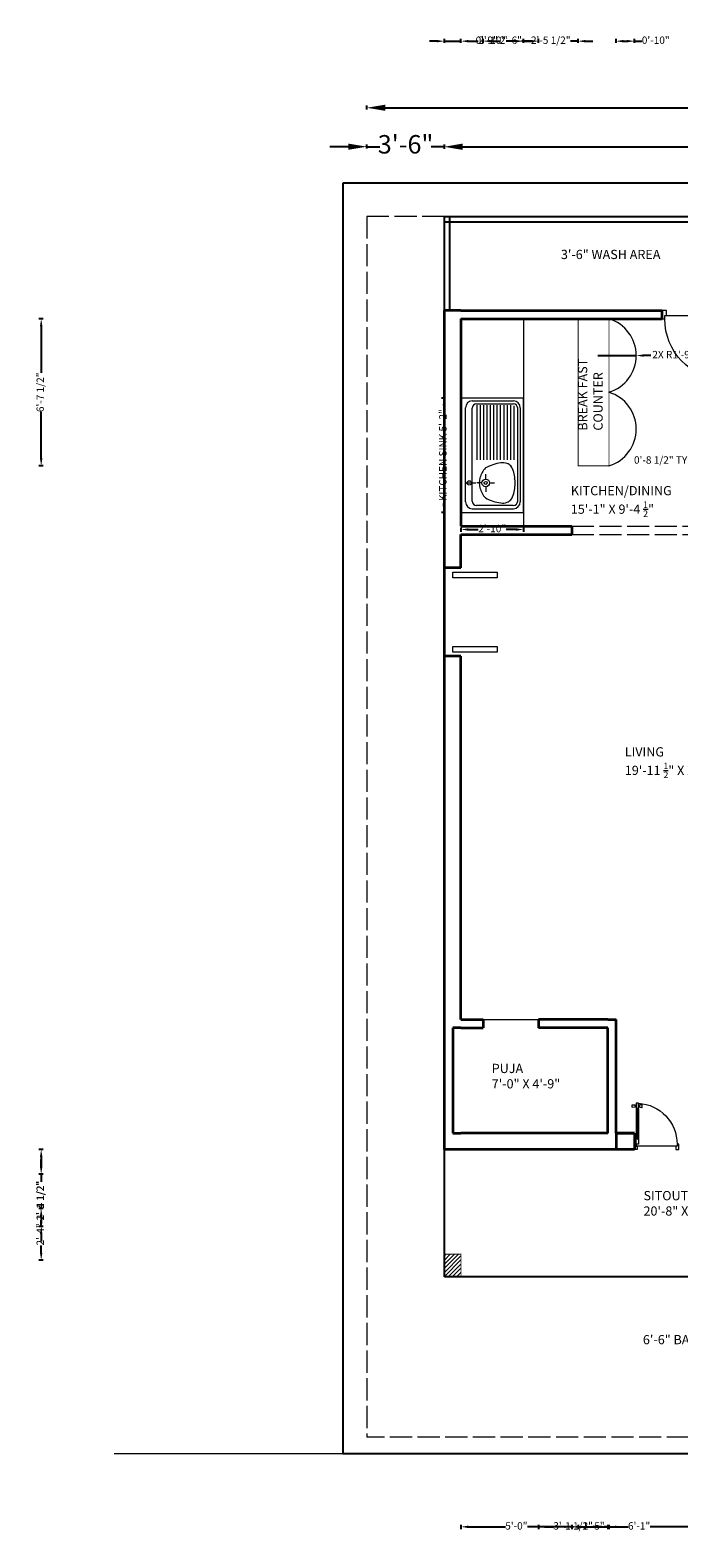
# Model space of a CAD drawing. Units: inches. Extents: x -638 to 186, y -762 to 59.
# Tile 1 of 31: x -638 to -287, y -759 to 59. Entities that reach past the tile are written whole.
import ezdxf

# ---------------------------------------------------------------- set-up
doc = ezdxf.new("R2010")
doc.units = ezdxf.units.IN
doc.linetypes.add('ACAD_ISO02W100', pattern=[15, 12, -3])
for name, color, linetype, lineweight in [('A-ANNO-DIMS', 2, 'Continuous', 18), ('A-AREA-IDEN', 1, 'Continuous', 18), ('A-COLS', 7, 'Continuous', 35), ('A-COLS-PATT', 1, 'Continuous', 13), ('A-DOOR', 3, 'Continuous', 18), ('A-FLOR-CASE', 1, 'Continuous', 18), ('A-FLOR-EDGE', 1, 'Continuous', 25), ('A-FLOR-FIXT', 9, 'Continuous', 18), ('A-FLOR-OVHD', 1, 'ACAD_ISO02W100', 18), ('A-WALL-OVHD', 1, 'ACAD_ISO02W100', 18), ('C-PROP', 7, 'Continuous', 25), ('C-ROAD', 7, 'Continuous', 18), ('txt', 7, 'Continuous', 18), ('wall', 7, 'Continuous', 35)]:
    doc.layers.add(name, color=color, linetype=linetype, lineweight=lineweight)
doc.styles.get("Standard").update_dxf_attribs({"font": 'arial.ttf'})
doc.dimstyles.new('ISO-25', dxfattribs={"dimtxt": 4, "dimasz": 4, "dimexe": 1.25, "dimexo": 0.625, "dimtad": 0, "dimlunit": 4, "dimtxsty": 'Standard', "dimcen": 2.5, "dimclrt": 256, "dimadec": 0, "dimazin": 0, "dimtfac": 1, "dimtmove": 0, "dimatfit": 3, "dimfxl": 1, "dimfxlon": 1, "dimarcsym": 0})

# ---------------------------------------------------------------- blocks, each defined once
blk = doc.blocks.new('19')
at = {"color": 0}
for p, q in [((4069.2, 13480.3), (4069.2, 13409.9)), ((4198.2, 13480.3), (4069.2, 13480.3)), ((4072.5, 13422.6), (4072.5, 13469.1)), ((4139, 13469.9), (4078.1, 13469.9)), ((4080.1, 13476.7), (4186.3, 13476.7)), ((4185.4, 13473.8), (4080.8, 13473.8)), ((4194, 13422.6), (4194, 13469.1)), ((4198.2, 13409.9), (4198.2, 13480.3)), ((4075.9, 13427.5), (4075.9, 13468.9)), ((4139, 13466), (4077.2, 13466)), ((4139, 13462.2), (4077.2, 13462.2)), ((4139, 13458.4), (4077.2, 13458.4)), ((4139, 13454.6), (4077.2, 13454.6)), ((4190.3, 13468.9), (4190.3, 13427.5)), ((4139, 13450.8), (4077.2, 13450.8)), ((4139, 13447), (4077.2, 13447)), ((4139, 13443.2), (4077.2, 13443.2)), ((4139, 13439.4), (4077.2, 13439.4)), ((4139, 13435.6), (4077.2, 13435.6)), ((4160.6, 13437.8), (4154.9, 13437.8)), ((4164.9, 13442.1), (4164.9, 13447.8)), ((4169.2, 13437.8), (4174.9, 13437.8)), ((4139, 13431.8), (4077.2, 13431.8)), ((4077.2, 13427.9), (4139, 13427.9)), ((4185.4, 13422.5), (4080.8, 13422.5)), ((4164.9, 13433.5), (4164.9, 13427.8)), ((4164.9, 13415.7), (4164.9, 13426.7)), ((4069.2, 13409.9), (4198.2, 13409.9)), ((4186.3, 13415), (4080.1, 13415))]:
    blk.add_line(p, q, dxfattribs=at)
for centre, radius in [((4164.9, 13437.8), 4.3), ((4164.9, 13437.8), 1.72), ((4164.9, 13419.2), 2.42)]:
    blk.add_circle(centre, radius, dxfattribs=at)
for points in [[(4080.1, 13476.7), (4075.9, 13476.7), (4072.5, 13473.3), (4072.5, 13469.1)], [(4080.8, 13473.8), (4078.1, 13473.8), (4075.9, 13471.6), (4075.9, 13468.9)], [(4160.4, 13470.6), (4155.2, 13470.4), (4150.2, 13468.9), (4145.7, 13466.1)], [(4162.1, 13470.8), (4161.6, 13470.7), (4161, 13470.6), (4160.5, 13470.4)], [(4169.4, 13470.6), (4167, 13471), (4164.6, 13471.1), (4162.1, 13470.8)], [(4184.1, 13466.1), (4179.7, 13468.9), (4174.6, 13470.4), (4169.4, 13470.6)], [(4190.3, 13468.9), (4190.3, 13471.6), (4188.1, 13473.8), (4185.4, 13473.8)], [(4194, 13469.1), (4194, 13473.3), (4190.5, 13476.7), (4186.3, 13476.7)], [(4143.1, 13461.8), (4142.2, 13459.6), (4141.9, 13457.2), (4142.4, 13454.9)], [(4142.4, 13454.9), (4143.2, 13448.8), (4145.1, 13442.9), (4148.1, 13437.5)], [(4145.7, 13466.1), (4144.5, 13464.9), (4143.6, 13463.4), (4143.1, 13461.8)], [(4181.8, 13437.5), (4184.8, 13442.9), (4186.7, 13448.8), (4187.5, 13454.9)], [(4186.7, 13461.8), (4186.2, 13463.4), (4185.3, 13464.9), (4184.1, 13466.1)], [(4187.5, 13454.9), (4187.9, 13457.2), (4187.7, 13459.6), (4186.7, 13461.8)], [(4148.1, 13437.5), (4151.2, 13434.5), (4155.1, 13432.4), (4159.3, 13431.3)], [(4170.6, 13431.3), (4174.8, 13432.4), (4178.7, 13434.5), (4181.8, 13437.5)], [(4072.5, 13422.6), (4072.5, 13418.4), (4075.9, 13415), (4080.1, 13415)], [(4075.9, 13427.5), (4075.9, 13424.7), (4078.1, 13422.5), (4080.8, 13422.5)], [(4159.3, 13431.3), (4163, 13430.2), (4166.9, 13430.2), (4170.6, 13431.3)], [(4185.4, 13422.5), (4188.1, 13422.5), (4190.3, 13424.7), (4190.3, 13427.5)], [(4186.3, 13415), (4190.5, 13415), (4194, 13418.4), (4194, 13422.6)]]:
    blk.add_open_spline(points, degree=3, dxfattribs=at)
blk = doc.blocks.new('*D8')
at = {"layer": 'A-ANNO-DIMS', "color": 0, "lineweight": -2, "transparency": 16777216}
for p, q in [((-465.53, -4.21), (-475.53, -4.21)), ((-455.53, -5.21), (-455.53, -2.96)), ((-455.53, -4.21), (-448.44, -4.21)), ((-413.53, -4.21), (-420.61, -4.21)), ((-413.53, -5.21), (-413.53, -2.96)), ((-403.53, -4.21), (-393.53, -4.21))]:
    blk.add_line(p, q, dxfattribs=at)
at = {"layer": 'A-ANNO-DIMS', "color": 0, "lineweight": 30, "transparency": 16777216}
for points in [[(-465.53, -2.54), (-465.53, -5.87), (-455.53, -4.21)], [(-403.53, -2.54), (-403.53, -5.87), (-413.53, -4.21)]]:
    blk.add_solid(points, dxfattribs=at)
at = {"layer": 'Defpoints', "color": 0, "lineweight": 30, "transparency": 16777216}
for p in [(-413.53, -4.21), (-455.53, -42.03), (-413.53, -42.03)]:
    blk.add_point(p, dxfattribs=at)
at = {"layer": 'A-ANNO-DIMS', "color": 0, "transparency": 16777216, "insert": (-434.53, -4.21), "char_height": 10, "attachment_point": 5}
blk.add_mtext('3\'-6"', dxfattribs=at)
blk = doc.blocks.new('*D9')
at = {"layer": 'A-ANNO-DIMS', "color": 0, "lineweight": -2, "transparency": 16777216}
for p, q in [((-413.53, -5.3), (-413.53, -3.05)), ((-403.53, -4.3), (-219.32, -4.3)), ((0.47, -4.3), (-183.73, -4.3)), ((10.47, -5.3), (10.47, -3.05))]:
    blk.add_line(p, q, dxfattribs=at)
at = {"layer": 'A-ANNO-DIMS', "color": 0, "lineweight": 30, "transparency": 16777216}
for points in [[(-403.53, -2.64), (-403.53, -5.97), (-413.53, -4.3)], [(0.47, -2.64), (0.47, -5.97), (10.47, -4.3)]]:
    blk.add_solid(points, dxfattribs=at)
at = {"layer": 'Defpoints', "color": 0, "lineweight": 30, "transparency": 16777216}
for p in [(10.47, -4.3), (-413.53, -42.03), (10.47, -42.03)]:
    blk.add_point(p, dxfattribs=at)
at = {"layer": 'A-ANNO-DIMS', "color": 0, "transparency": 16777216, "insert": (-201.53, -4.3), "char_height": 10, "attachment_point": 5}
blk.add_mtext('35\'-4"', dxfattribs=at)
blk = doc.blocks.new('*D11')
at = {"layer": 'A-ANNO-DIMS', "color": 0, "lineweight": -2, "transparency": 16777216}
for p, q in [((-455.53, 15.89), (-455.53, 18.14)), ((-445.53, 16.89), (-231.53, 16.89)), ((18.47, 16.89), (-195.52, 16.89)), ((28.47, 15.89), (28.47, 18.14))]:
    blk.add_line(p, q, dxfattribs=at)
at = {"layer": 'A-ANNO-DIMS', "color": 0, "lineweight": 30, "transparency": 16777216}
for points in [[(-445.53, 18.56), (-445.53, 15.23), (-455.53, 16.89)], [(18.47, 18.56), (18.47, 15.23), (28.47, 16.89)]]:
    blk.add_solid(points, dxfattribs=at)
at = {"layer": 'Defpoints', "color": 0, "lineweight": 30, "transparency": 16777216}
for p in [(28.47, 16.89), (-455.53, -42.03), (28.47, -42.03)]:
    blk.add_point(p, dxfattribs=at)
at = {"layer": 'A-ANNO-DIMS', "color": 0, "transparency": 16777216, "insert": (-213.53, 16.89), "char_height": 10, "attachment_point": 5}
blk.add_mtext('40\'-4"', dxfattribs=at)
blk = doc.blocks.new('DOOR-SWING-36IN')
for p, q in [((35.54, 35.1), (4.05, 35.09)), ((3.16, 4.5), (3.16, 28.79)), ((3.95, 4.05), (3.94, 29.24)), ((4.06, 4.05), (4.06, 29.24)), ((4.18, 4.05), (4.17, 29.24)), ((4.96, 4.5), (4.96, 28.79))]:
    blk.add_line(p, q)
for points in [[(3.16, 33.29), (3.15, 35.09), (4.05, 35.09), (4.05, 37.78), (1.8, 37.78), (1.81, 33.29), (3.16, 33.29)], [(4.28, 28.79), (4.96, 28.79), (4.95, 33.29), (3.16, 33.29), (3.16, 28.79), (3.83, 28.79), (3.83, 29.24), (4.28, 29.24), (4.28, 28.79)], [(36.44, 33.3), (36.44, 35.1), (35.54, 35.1), (35.54, 37.79), (37.79, 37.8), (37.79, 33.3), (36.44, 33.3)], [(4.29, 4.5), (4.96, 4.5), (4.96, 0), (3.17, 0), (3.16, 4.5), (3.84, 4.5), (3.84, 4.05), (4.29, 4.05), (4.29, 4.5)]]:
    blk.add_lwpolyline(points)
for points in [[(2.05, 3.17), (0.25, 3.35, 0.443716), (0, 3.12), (0, 1.37, 0.443716), (0.25, 1.15), (2.05, 1.33, 0.385314), (2.25, 1.55), (2.25, 2.94, 0.385314)], [(6.08, 3.17), (7.88, 3.35, -0.443716), (8.13, 3.13), (8.13, 1.37, -0.443716), (7.88, 1.15), (6.08, 1.33, -0.385314), (5.88, 1.55), (5.88, 2.95, -0.385314)]]:
    blk.add_lwpolyline(points, format="xyb", close=True)
for points in [[(3.16, 2.47), (2.25, 2.47), (2.25, 2.02), (3.17, 2.02)], [(4.96, 2.47), (5.88, 2.47), (5.88, 2.03), (4.96, 2.02)]]:
    blk.add_lwpolyline(points, close=True)
for centre, radius, start, end in [((3.06, 33.32), 33.38, 273.26531, 359.95298), ((3.92, 28.83), 0.371, 186.45223, 273.3078), ((4.19, 28.83), 0.371, 266.72821, 353.58377), ((3.93, 4.46), 0.371, 86.72821, 173.58377), ((4.2, 4.46), 0.371, 6.45223, 93.3078)]:
    blk.add_arc(centre, radius, start, end)
blk = doc.blocks.new('DOOR-ENTRY-24IN-LEAF')
for p, q in [((21.85, 22.14), (21.85, 5.99)), ((22.38, 22.44), (22.37, 5.69)), ((22.45, 22.44), (22.45, 5.69)), ((22.53, 22.44), (22.52, 5.69)), ((23.05, 22.14), (23.04, 5.99)), ((1.5, 1.8), (22.44, 1.8))]:
    blk.add_line(p, q)
for points in [[(22.3, 22.14), (21.85, 22.14), (21.85, 25.14), (23.05, 25.14), (23.05, 22.14), (22.6, 22.14), (22.6, 22.44), (22.3, 22.44), (22.3, 22.14)], [(0.9, 3), (0.9, 1.8), (1.5, 1.8), (1.5, 0.01), (0, 0.01), (0, 3), (0.9, 3)], [(22.3, 5.99), (21.85, 5.99), (21.85, 2.99), (23.04, 2.99), (23.04, 5.99), (22.59, 5.99), (22.59, 5.69), (22.3, 5.69), (22.3, 5.99)], [(23.04, 2.99), (23.04, 1.8), (22.44, 1.8), (22.44, 0), (23.94, 0), (23.94, 2.99), (23.04, 2.99)]]:
    blk.add_lwpolyline(points)
for points in [[(21.11, 23.03), (19.91, 22.91, -0.443716), (19.75, 23.06), (19.75, 24.22, -0.443716), (19.91, 24.37), (21.11, 24.25, -0.385314), (21.24, 24.1), (21.24, 23.18, -0.385314)], [(23.79, 23.03), (24.99, 22.91, 0.443716), (25.15, 23.06), (25.16, 24.22, 0.443716), (24.99, 24.37), (23.79, 24.25, 0.385314), (23.66, 24.1), (23.66, 23.18, 0.385314)]]:
    blk.add_lwpolyline(points, format="xyb", close=True)
for points in [[(21.85, 23.49), (21.24, 23.49), (21.24, 23.79), (21.85, 23.79)], [(23.05, 23.49), (23.66, 23.49), (23.66, 23.79), (23.05, 23.79)]]:
    blk.add_lwpolyline(points, close=True)
for centre, radius, start, end in [((23.1, 2.97), 22.21, 93.2293, 179.91697), ((22.36, 22.17), 0.247, 186.41623, 273.27179), ((22.54, 22.17), 0.247, 266.6922, 353.54777), ((22.36, 5.96), 0.247, 86.6922, 173.54777), ((22.53, 5.96), 0.247, 6.41623, 93.27179)]:
    blk.add_arc(centre, radius, start, end)
blk = doc.blocks.new('*D22')
at = {"layer": 'A-ANNO-DIMS', "color": 0, "lineweight": -2, "transparency": 16777216}
for p, q in [((-272.41, -174.6), (-276.41, -174.6)), ((-268.41, -173.71), (-268.41, -175.85)), ((-260.07, -174.6), (-268.41, -174.6)), ((-260.07, -173.71), (-260.07, -175.85)), ((-256.07, -174.6), (-252.07, -174.6))]:
    blk.add_line(p, q, dxfattribs=at)
at = {"layer": 'A-ANNO-DIMS', "color": 0, "lineweight": 30, "transparency": 16777216}
for points in [[(-272.41, -173.93), (-272.41, -175.26), (-268.41, -174.6)], [(-256.07, -173.93), (-256.07, -175.26), (-260.07, -174.6)]]:
    blk.add_solid(points, dxfattribs=at)
at = {"layer": 'Defpoints', "color": 0, "lineweight": 30, "transparency": 16777216}
for p in [(-268.41, -173.09), (-268.41, -174.6), (-260.07, -173.09)]:
    blk.add_point(p, dxfattribs=at)
at = {"layer": 'A-ANNO-DIMS', "transparency": 16777216, "insert": (-293.89, -174.6), "char_height": 4, "attachment_point": 5, "rotation": 360}
blk.add_mtext('0\'-8 1/2" TYP.', dxfattribs=at)
blk = doc.blocks.new('*D33')
at = {"layer": 'A-ANNO-DIMS', "color": 0, "lineweight": -2, "transparency": 16777216}
for p, q in [((-412.83, -140.48), (-415.08, -140.48)), ((-413.83, -144.48), (-413.83, -145.3)), ((-412.83, -202.49), (-415.08, -202.49)), ((-413.83, -198.49), (-413.83, -197.68))]:
    blk.add_line(p, q, dxfattribs=at)
at = {"layer": 'A-ANNO-DIMS', "color": 0, "lineweight": 30, "transparency": 16777216}
for points in [[(-414.49, -144.48), (-413.16, -144.48), (-413.83, -140.48)], [(-414.49, -198.49), (-413.16, -198.49), (-413.83, -202.49)]]:
    blk.add_solid(points, dxfattribs=at)
at = {"layer": 'Defpoints', "color": 0, "lineweight": 30, "transparency": 16777216}
for p in [(-404.53, -140.48), (-413.83, -202.49), (-404.53, -202.49)]:
    blk.add_point(p, dxfattribs=at)
at = {"layer": 'A-ANNO-DIMS', "transparency": 16777216, "insert": (-413.83, -171.49), "char_height": 4, "attachment_point": 5, "rotation": 90}
blk.add_mtext('KITCHEN SINK 5\'-2"', dxfattribs=at)
blk = doc.blocks.new('*D34')
at = {"layer": 'A-ANNO-DIMS', "color": 0, "lineweight": -2, "transparency": 16777216}
for p, q in [((-404.53, -210.79), (-404.53, -213.04)), ((-400.53, -211.79), (-395.15, -211.79)), ((-374.71, -211.79), (-380.09, -211.79)), ((-370.71, -210.79), (-370.71, -213.04))]:
    blk.add_line(p, q, dxfattribs=at)
at = {"layer": 'A-ANNO-DIMS', "color": 0, "lineweight": 30, "transparency": 16777216}
for points in [[(-400.53, -211.12), (-400.53, -212.46), (-404.53, -211.79)], [(-374.71, -211.12), (-374.71, -212.46), (-370.71, -211.79)]]:
    blk.add_solid(points, dxfattribs=at)
at = {"layer": 'Defpoints', "color": 0, "lineweight": 30, "transparency": 16777216}
for p in [(-404.53, -202.49), (-370.71, -202.49), (-370.71, -211.79)]:
    blk.add_point(p, dxfattribs=at)
at = {"layer": 'A-ANNO-DIMS', "transparency": 16777216, "insert": (-387.62, -211.79), "char_height": 4, "attachment_point": 5}
blk.add_mtext('2\'-10"', dxfattribs=at)
blk = doc.blocks.new('*D37')
at = {"layer": 'A-ANNO-DIMS', "color": 0, "lineweight": -2, "transparency": 16777216}
for p, q in [((182.66, -232.53), (184.91, -232.53)), ((183.66, -236.53), (183.66, -250.51)), ((183.66, -276.53), (183.66, -262.56)), ((182.66, -280.53), (184.91, -280.53))]:
    blk.add_line(p, q, dxfattribs=at)
at = {"layer": 'A-ANNO-DIMS', "color": 0, "lineweight": 30, "transparency": 16777216}
for points in [[(183, -236.53), (184.33, -236.53), (183.66, -232.53)], [(183, -276.53), (184.33, -276.53), (183.66, -280.53)]]:
    blk.add_solid(points, dxfattribs=at)
at = {"layer": 'Defpoints', "color": 0, "lineweight": 30, "transparency": 16777216}
for p in [(-404.53, -232.53), (-404.53, -280.53), (183.66, -280.53)]:
    blk.add_point(p, dxfattribs=at)
at = {"layer": 'A-ANNO-DIMS', "transparency": 16777216, "insert": (183.66, -256.53), "char_height": 4, "attachment_point": 5, "rotation": 90}
blk.add_mtext('4\'-0"', dxfattribs=at)
blk = doc.blocks.new('*D38')
at = {"layer": 'A-ANNO-DIMS', "color": 0, "lineweight": -2, "transparency": 16777216}
for p, q in [((182.66, -280.53), (184.91, -280.53)), ((183.66, -284.53), (183.66, -371.73)), ((183.66, -473.53), (183.66, -386.34)), ((182.66, -477.53), (184.91, -477.53))]:
    blk.add_line(p, q, dxfattribs=at)
at = {"layer": 'A-ANNO-DIMS', "color": 0, "lineweight": 30, "transparency": 16777216}
for points in [[(183, -284.53), (184.33, -284.53), (183.66, -280.53)], [(183, -473.53), (184.33, -473.53), (183.66, -477.53)]]:
    blk.add_solid(points, dxfattribs=at)
at = {"layer": 'Defpoints', "color": 0, "lineweight": 30, "transparency": 16777216}
for p in [(-404.53, -280.53), (-404.53, -477.53), (183.66, -477.53)]:
    blk.add_point(p, dxfattribs=at)
at = {"layer": 'A-ANNO-DIMS', "transparency": 16777216, "insert": (183.66, -379.03), "char_height": 4, "attachment_point": 5, "rotation": 90}
blk.add_mtext('16\'-5"', dxfattribs=at)
blk = doc.blocks.new('*D39')
at = {"layer": 'A-ANNO-DIMS', "color": 0, "lineweight": -2, "transparency": 16777216}
for p, q in [((-344.53, -751.58), (-344.53, -753.83)), ((-271.53, -751.58), (-271.53, -753.83)), ((-340.53, -752.58), (-313.98, -752.58)), ((-275.53, -752.58), (-302.07, -752.58))]:
    blk.add_line(p, q, dxfattribs=at)
at = {"layer": 'A-ANNO-DIMS', "color": 0, "lineweight": 30, "transparency": 16777216}
for points in [[(-340.53, -751.92), (-340.53, -753.25), (-344.53, -752.58)], [(-275.53, -751.92), (-275.53, -753.25), (-271.53, -752.58)]]:
    blk.add_solid(points, dxfattribs=at)
at = {"layer": 'Defpoints', "color": 0, "lineweight": 30, "transparency": 16777216}
for p in [(-344.53, -214.53), (-271.53, -214.53), (-271.53, -752.58)]:
    blk.add_point(p, dxfattribs=at)
at = {"layer": 'A-ANNO-DIMS', "transparency": 16777216, "insert": (-308.03, -752.58), "char_height": 4, "attachment_point": 5}
blk.add_mtext('6\'-1"', dxfattribs=at)
blk = doc.blocks.new('*D40')
at = {"layer": 'A-ANNO-DIMS', "color": 0, "lineweight": -2, "transparency": 16777216}
for p, q in [((-404.53, -751.58), (-404.53, -753.83)), ((-344.53, -751.58), (-344.53, -753.83)), ((-400.53, -752.58), (-380.47, -752.58)), ((-348.53, -752.58), (-368.58, -752.58))]:
    blk.add_line(p, q, dxfattribs=at)
at = {"layer": 'A-ANNO-DIMS', "color": 0, "lineweight": 30, "transparency": 16777216}
for points in [[(-400.53, -751.92), (-400.53, -753.25), (-404.53, -752.58)], [(-348.53, -751.92), (-348.53, -753.25), (-344.53, -752.58)]]:
    blk.add_solid(points, dxfattribs=at)
at = {"layer": 'Defpoints', "color": 0, "lineweight": 30, "transparency": 16777216}
for p in [(-404.53, -214.53), (-344.53, -214.53), (-344.53, -752.58)]:
    blk.add_point(p, dxfattribs=at)
at = {"layer": 'A-ANNO-DIMS', "transparency": 16777216, "insert": (-374.53, -752.58), "char_height": 4, "attachment_point": 5}
blk.add_mtext('5\'-0"', dxfattribs=at)
blk = doc.blocks.new('*D41')
at = {"layer": 'A-ANNO-DIMS', "color": 0, "lineweight": -2, "transparency": 16777216}
for p, q in [((-392.53, 52.02), (-392.53, 54.27)), ((-388.53, 53.02), (-383.5, 53.02)), ((-366.53, 53.02), (-371.55, 53.02)), ((-362.53, 52.02), (-362.53, 54.27))]:
    blk.add_line(p, q, dxfattribs=at)
at = {"layer": 'A-ANNO-DIMS', "color": 0, "lineweight": 30, "transparency": 16777216}
for points in [[(-388.53, 53.68), (-388.53, 52.35), (-392.53, 53.02)], [(-366.53, 53.68), (-366.53, 52.35), (-362.53, 53.02)]]:
    blk.add_solid(points, dxfattribs=at)
at = {"layer": 'Defpoints', "color": 0, "lineweight": 30, "transparency": 16777216}
for p in [(-362.53, 53.02), (-392.53, -477.53), (-362.53, -477.53)]:
    blk.add_point(p, dxfattribs=at)
at = {"layer": 'A-ANNO-DIMS', "transparency": 16777216, "insert": (-377.53, 53.02), "char_height": 4, "attachment_point": 5}
blk.add_mtext('2\'-6"', dxfattribs=at)
blk = doc.blocks.new('*D42')
at = {"layer": 'A-ANNO-DIMS', "color": 0, "lineweight": -2, "transparency": 16777216}
for p, q in [((-362.53, -751.58), (-362.53, -753.83)), ((-325.03, -751.58), (-325.03, -753.83)), ((-358.53, -752.58), (-354.38, -752.58)), ((-329.03, -752.58), (-333.18, -752.58))]:
    blk.add_line(p, q, dxfattribs=at)
at = {"layer": 'A-ANNO-DIMS', "color": 0, "lineweight": 30, "transparency": 16777216}
for points in [[(-358.53, -751.92), (-358.53, -753.25), (-362.53, -752.58)], [(-329.03, -751.92), (-329.03, -753.25), (-325.03, -752.58)]]:
    blk.add_solid(points, dxfattribs=at)
at = {"layer": 'Defpoints', "color": 0, "lineweight": 30, "transparency": 16777216}
for p in [(-362.53, -482.03), (-325.03, -482.03), (-325.03, -752.58)]:
    blk.add_point(p, dxfattribs=at)
at = {"layer": 'A-ANNO-DIMS', "transparency": 16777216, "insert": (-343.78, -752.58), "char_height": 4, "attachment_point": 5}
blk.add_mtext('3\'-1 1/2"', dxfattribs=at)
blk = doc.blocks.new('*D43')
at = {"layer": 'A-ANNO-DIMS', "color": 0, "lineweight": -2, "transparency": 16777216}
for p, q in [((-320.53, 52.02), (-320.53, 54.27)), ((-316.53, 53.02), (-314.53, 53.02)), ((-310.53, 52.02), (-310.53, 54.27)), ((-310.53, 53.02), (-306.53, 53.02))]:
    blk.add_line(p, q, dxfattribs=at)
at = {"layer": 'A-ANNO-DIMS', "color": 0, "lineweight": 30, "transparency": 16777216}
for points in [[(-316.53, 53.68), (-316.53, 52.35), (-320.53, 53.02)], [(-314.53, 53.68), (-314.53, 52.35), (-310.53, 53.02)]]:
    blk.add_solid(points, dxfattribs=at)
at = {"layer": 'Defpoints', "color": 0, "lineweight": 30, "transparency": 16777216}
for p in [(-310.53, 53.02), (-320.53, -539.03), (-310.53, -539.03)]:
    blk.add_point(p, dxfattribs=at)
at = {"layer": 'A-ANNO-DIMS', "transparency": 16777216, "insert": (-299.03, 53.02), "char_height": 4, "attachment_point": 5}
blk.add_mtext('0\'-10"', dxfattribs=at)
blk = doc.blocks.new('*D44')
at = {"layer": 'A-ANNO-DIMS', "color": 0, "lineweight": -2, "transparency": 16777216}
for p, q in [((-417.53, 53.02), (-421.53, 53.02)), ((-413.53, 52.02), (-413.53, 54.27)), ((-413.53, 53.02), (-404.53, 53.02)), ((-404.53, 52.02), (-404.53, 54.27)), ((-400.53, 53.02), (-396.53, 53.02))]:
    blk.add_line(p, q, dxfattribs=at)
at = {"layer": 'A-ANNO-DIMS', "color": 0, "lineweight": 30, "transparency": 16777216}
for points in [[(-417.53, 53.68), (-417.53, 52.35), (-413.53, 53.02)], [(-400.53, 53.68), (-400.53, 52.35), (-404.53, 53.02)]]:
    blk.add_solid(points, dxfattribs=at)
at = {"layer": 'Defpoints', "color": 0, "lineweight": 30, "transparency": 16777216}
for p in [(-404.53, 53.02), (-413.53, -93.03), (-404.53, -97.53)]:
    blk.add_point(p, dxfattribs=at)
at = {"layer": 'A-ANNO-DIMS', "transparency": 16777216, "insert": (-390.58, 53.02), "char_height": 4, "attachment_point": 5}
blk.add_mtext('0\'-9"', dxfattribs=at)
blk = doc.blocks.new('*D45')
at = {"layer": 'A-ANNO-DIMS', "color": 0, "lineweight": -2, "transparency": 16777216}
for p, q in [((-374.7, 53.02), (-378.7, 53.02)), ((-370.7, 52.02), (-370.7, 54.27)), ((-370.7, 53.02), (-366.54, 53.02)), ((-341.11, 53.02), (-345.27, 53.02)), ((-341.11, 52.02), (-341.11, 54.27)), ((-337.11, 53.02), (-333.11, 53.02))]:
    blk.add_line(p, q, dxfattribs=at)
at = {"layer": 'A-ANNO-DIMS', "color": 0, "lineweight": 30, "transparency": 16777216}
for points in [[(-374.7, 53.68), (-374.7, 52.35), (-370.7, 53.02)], [(-337.11, 53.68), (-337.11, 52.35), (-341.11, 53.02)]]:
    blk.add_solid(points, dxfattribs=at)
at = {"layer": 'Defpoints', "color": 0, "lineweight": 30, "transparency": 16777216}
for p in [(-341.11, 53.02), (-370.7, -97.53), (-341.11, -97.53)]:
    blk.add_point(p, dxfattribs=at)
at = {"layer": 'A-ANNO-DIMS', "transparency": 16777216, "insert": (-355.9, 53.02), "char_height": 4, "attachment_point": 5}
blk.add_mtext('2\'-5 1/2"', dxfattribs=at)
blk = doc.blocks.new('*D46')
at = {"layer": 'A-ANNO-DIMS', "color": 0, "lineweight": -2, "transparency": 16777216}
for p, q in [((-630.93, -97.53), (-633.18, -97.53)), ((-631.93, -101.53), (-631.93, -126.78)), ((-631.93, -173.25), (-631.93, -148)), ((-630.93, -177.25), (-633.18, -177.25))]:
    blk.add_line(p, q, dxfattribs=at)
at = {"layer": 'A-ANNO-DIMS', "color": 0, "lineweight": 30, "transparency": 16777216}
for points in [[(-632.59, -101.53), (-631.26, -101.53), (-631.93, -97.53)], [(-632.59, -173.25), (-631.26, -173.25), (-631.93, -177.25)]]:
    blk.add_solid(points, dxfattribs=at)
at = {"layer": 'Defpoints', "color": 0, "lineweight": 30, "transparency": 16777216}
for p in [(-341.11, -97.53), (-631.93, -177.25), (-341.11, -177.25)]:
    blk.add_point(p, dxfattribs=at)
at = {"layer": 'A-ANNO-DIMS', "transparency": 16777216, "insert": (-631.93, -137.39), "char_height": 4, "attachment_point": 5, "rotation": 90}
blk.add_mtext('6\'-7 1/2"', dxfattribs=at)
blk = doc.blocks.new('*D47')
at = {"layer": 'A-ANNO-DIMS', "color": 0, "lineweight": -2, "transparency": 16777216}
for p, q in [((-341.11, -751.58), (-341.11, -753.83)), ((-324.35, -751.58), (-324.35, -753.83)), ((-345.11, -752.58), (-349.11, -752.58)), ((-341.11, -752.58), (-338.48, -752.58)), ((-324.35, -752.58), (-326.97, -752.58)), ((-320.35, -752.58), (-316.35, -752.58))]:
    blk.add_line(p, q, dxfattribs=at)
at = {"layer": 'A-ANNO-DIMS', "color": 0, "lineweight": 30, "transparency": 16777216}
for points in [[(-345.11, -751.92), (-345.11, -753.25), (-341.11, -752.58)], [(-320.35, -751.92), (-320.35, -753.25), (-324.35, -752.58)]]:
    blk.add_solid(points, dxfattribs=at)
at = {"layer": 'Defpoints', "color": 0, "lineweight": 30, "transparency": 16777216}
for p in [(-341.11, -177.25), (-324.35, -177.25), (-324.35, -752.58)]:
    blk.add_point(p, dxfattribs=at)
at = {"layer": 'A-ANNO-DIMS', "transparency": 16777216, "insert": (-332.73, -752.58), "char_height": 4, "attachment_point": 5}
blk.add_mtext('1\'-5"', dxfattribs=at)
blk = doc.blocks.new('*D50')
at = {"layer": 'A-ANNO-DIMS', "color": 0, "lineweight": -2, "transparency": 16777216}
for p, q in [((-631.93, -557.43), (-631.93, -553.43)), ((-630.93, -561.43), (-633.18, -561.43)), ((-631.93, -561.43), (-631.93, -564.98)), ((-631.93, -589.8), (-631.93, -586.25)), ((-630.93, -589.8), (-633.18, -589.8)), ((-631.93, -593.8), (-631.93, -597.8))]:
    blk.add_line(p, q, dxfattribs=at)
at = {"layer": 'A-ANNO-DIMS', "color": 0, "lineweight": 30, "transparency": 16777216}
for points in [[(-632.59, -557.43), (-631.26, -557.43), (-631.93, -561.43)], [(-632.59, -593.8), (-631.26, -593.8), (-631.93, -589.8)]]:
    blk.add_solid(points, dxfattribs=at)
at = {"layer": 'Defpoints', "color": 0, "lineweight": 30, "transparency": 16777216}
for p in [(-156.03, -561.43), (-631.93, -589.8), (-156.03, -589.8)]:
    blk.add_point(p, dxfattribs=at)
at = {"layer": 'A-ANNO-DIMS', "transparency": 16777216, "insert": (-631.93, -575.62), "char_height": 4, "attachment_point": 5, "rotation": 90}
blk.add_mtext('2\'-4 1/2"', dxfattribs=at)
blk = doc.blocks.new('*D52')
at = {"layer": 'A-ANNO-DIMS', "color": 0, "lineweight": -2, "transparency": 16777216}
for p, q in [((-630.93, -580.03), (-633.18, -580.03)), ((-631.93, -584.03), (-631.93, -588.06)), ((-631.93, -604.03), (-631.93, -600.01)), ((-630.93, -608.03), (-633.18, -608.03))]:
    blk.add_line(p, q, dxfattribs=at)
at = {"layer": 'A-ANNO-DIMS', "color": 0, "lineweight": 30, "transparency": 16777216}
for points in [[(-632.59, -584.03), (-631.26, -584.03), (-631.93, -580.03)], [(-632.59, -604.03), (-631.26, -604.03), (-631.93, -608.03)]]:
    blk.add_solid(points, dxfattribs=at)
at = {"layer": 'Defpoints', "color": 0, "lineweight": 30, "transparency": 16777216}
for p in [(-29.91, -580.03), (-631.93, -608.03), (-40.41, -608.03)]:
    blk.add_point(p, dxfattribs=at)
at = {"layer": 'A-ANNO-DIMS', "transparency": 16777216, "insert": (-631.93, -594.03), "char_height": 4, "attachment_point": 5, "rotation": 90}
blk.add_mtext('2\'-4"', dxfattribs=at)
blk = doc.blocks.new('*D54')
at = {"layer": 'A-ANNO-DIMS', "color": 0, "lineweight": -2, "transparency": 16777216}
for p, q in [((-404.53, 52.02), (-404.53, 54.27)), ((-400.53, 53.02), (-395.14, 53.02)), ((-374.7, 53.02), (-380.08, 53.02)), ((-370.7, 52.02), (-370.7, 54.27))]:
    blk.add_line(p, q, dxfattribs=at)
at = {"layer": 'A-ANNO-DIMS', "color": 0, "lineweight": 30, "transparency": 16777216}
for points in [[(-400.53, 53.68), (-400.53, 52.35), (-404.53, 53.02)], [(-374.7, 53.68), (-374.7, 52.35), (-370.7, 53.02)]]:
    blk.add_solid(points, dxfattribs=at)
at = {"layer": 'Defpoints', "color": 0, "lineweight": 30, "transparency": 16777216}
for p in [(-370.7, 53.02), (-404.53, -97.53), (-370.7, -97.53)]:
    blk.add_point(p, dxfattribs=at)
at = {"layer": 'A-ANNO-DIMS', "transparency": 16777216, "insert": (-387.61, 53.02), "char_height": 4, "attachment_point": 5}
blk.add_mtext('2\'-10"', dxfattribs=at)
blk = doc.blocks.new('*D57')
at = {"layer": 'A-ANNO-DIMS', "color": 0, "lineweight": -2, "transparency": 16777216}
for p, q in [((-630.93, -548.03), (-633.18, -548.03)), ((-631.93, -552.03), (-631.93, -557.43)), ((-630.93, -561.43), (-633.18, -561.43)), ((-631.93, -561.43), (-631.93, -565.43))]:
    blk.add_line(p, q, dxfattribs=at)
at = {"layer": 'A-ANNO-DIMS', "color": 0, "lineweight": 30, "transparency": 16777216}
for points in [[(-632.59, -552.03), (-631.26, -552.03), (-631.93, -548.03)], [(-632.59, -557.43), (-631.26, -557.43), (-631.93, -561.43)]]:
    blk.add_solid(points, dxfattribs=at)
at = {"layer": 'Defpoints', "color": 0, "lineweight": 30, "transparency": 16777216}
for p in [(-156.03, -548.03), (-631.93, -561.43), (-156.03, -561.43)]:
    blk.add_point(p, dxfattribs=at)
at = {"layer": 'A-ANNO-DIMS', "transparency": 16777216, "insert": (-631.93, -575.84), "char_height": 4, "attachment_point": 5, "rotation": 90}
blk.add_mtext('1\'-1 1/2"', dxfattribs=at)
blk = doc.blocks.new('*D58')
at = {"layer": 'A-ANNO-DIMS', "color": 0, "lineweight": -2, "transparency": 16777216}
for p, q in [((-330.45, -117.46), (-309.6, -117.46)), ((-301.6, -117.46), (-305.6, -117.46))]:
    blk.add_line(p, q, dxfattribs=at)
at = {"layer": 'A-ANNO-DIMS', "color": 0, "lineweight": 30, "transparency": 16777216}
blk.add_solid([(-305.6, -116.8), (-305.6, -118.13), (-309.6, -117.46)], dxfattribs=at)
at = {"layer": 'Defpoints', "color": 0, "lineweight": 30, "transparency": 16777216}
for p in [(-330.45, -117.46), (-309.6, -117.46)]:
    blk.add_point(p, dxfattribs=at)
at = {"layer": 'A-ANNO-DIMS', "transparency": 16777216, "insert": (-289.42, -117.46), "char_height": 4, "attachment_point": 5, "rotation": 0.00132}
blk.add_mtext('2X R1\'-9"', dxfattribs=at)

msp = doc.modelspace()

# ---------------------------------------------------------------- hatches: boundary and pattern name
at = {"layer": 'A-COLS-PATT'}
h = msp.add_hatch(dxfattribs=at)
h.set_pattern_fill('ANSI31', color=256, scale=0.5)
h.set_pattern_definition([(45, (-922.1772, 71.0805), (-1.122532, 1.122532), [])])
h.paths.add_polyline_path([(-413.526, -604.707), (-413.526, -616.707), (-404.526, -616.707), (-404.526, -604.707)])

# ---------------------------------------------------------------- linework, layer by layer
at = {"layer": 'A-COLS', "const_width": 0.5}
msp.add_lwpolyline([(-413.526, -604.707), (-404.526, -604.707), (-404.526, -616.707), (-413.526, -616.707)], close=True, dxfattribs=at)
at = {"layer": 'A-DOOR'}
msp.add_line((-392.526, -477.533), (-362.526, -477.533), dxfattribs=at)
at = {"layer": 'A-FLOR-CASE'}
msp.add_line((-370.702, -97.533), (-370.702, -210.033), dxfattribs=at)
at = {"layer": 'A-FLOR-CASE', "const_width": 0.5}
msp.add_lwpolyline([(-341.107, -97.533), (-324.346, -97.533), (-324.346, -177.25), (-341.107, -177.25)], close=True, dxfattribs=at)
at = {"layer": 'A-FLOR-CASE'}
for points in [[(-408.938, -235.008), (-384.938, -235.008), (-384.938, -238.008), (-408.938, -238.008)], [(-408.938, -275.281), (-384.938, -275.281), (-384.938, -278.281), (-408.938, -278.281)]]:
    msp.add_lwpolyline(points, close=True, dxfattribs=at)
for centre in [(-330.447, -117.462), (-330.447, -157.321)]:
    msp.add_arc(centre, 20.842, 287.02147, 72.97853, dxfattribs=at)
at = {"layer": 'A-FLOR-EDGE'}
for p, q in [((-413.526, -42.033), (-223.526, -42.033)), ((-413.526, -93.033), (-413.526, -42.033)), ((-413.526, -45.033), (-223.526, -45.033)), ((-410.526, -93.033), (-410.526, -42.033)), ((-413.526, -617.033), (-413.526, -548.033)), ((-165.026, -617.033), (-413.526, -617.033))]:
    msp.add_line(p, q, dxfattribs=at)
at = {"layer": 'A-FLOR-OVHD'}
for p, q in [((-413.526, -42.033), (-455.526, -42.033)), ((-455.526, -42.033), (-455.526, -704.033)), ((-116.044, -704.033), (-455.526, -704.033))]:
    msp.add_line(p, q, dxfattribs=at)
at = {"layer": 'A-WALL-OVHD'}
for p, q in [((-344.526, -210.033), (-271.526, -210.033)), ((-344.526, -214.533), (-271.526, -214.533))]:
    msp.add_line(p, q, dxfattribs=at)
at = {"layer": 'C-PROP'}
for p, q in [((10.474, -24.033), (-468.465, -24.033)), ((-468.465, -24.033), (-468.465, -713.033)), ((-455.526, -713.033), (-468.465, -713.033)), ((-116.044, -713.033), (-455.526, -713.033))]:
    msp.add_line(p, q, dxfattribs=at)
at = {"layer": 'C-ROAD'}
msp.add_line((-468.465, -713.033), (-592.376, -713.033), dxfattribs=at)
at = {"layer": 'wall'}
for p, q in [((-404.526, -93.033), (-413.526, -93.033)), ((-413.526, -232.533), (-413.526, -93.033)), ((-404.526, -93.033), (-295.526, -93.033)), ((-404.526, -97.533), (-295.526, -97.533)), ((-404.526, -97.533), (-404.526, -210.033)), ((-295.526, -97.533), (-295.526, -93.033)), ((-404.526, -210.033), (-344.526, -210.033)), ((-344.526, -210.033), (-344.526, -214.533)), ((-404.526, -214.533), (-344.526, -214.533)), ((-404.526, -232.533), (-404.526, -214.533)), ((-404.526, -232.533), (-413.526, -232.533)), ((-413.526, -280.533), (-413.526, -232.533)), ((-404.526, -280.533), (-413.526, -280.533)), ((-413.526, -548.033), (-413.526, -280.533)), ((-404.526, -477.533), (-404.526, -280.533)), ((-404.526, -482.033), (-409.026, -482.033)), ((-409.026, -482.033), (-409.026, -539.033)), ((-404.526, -477.533), (-392.526, -477.533)), ((-404.526, -482.033), (-392.526, -482.033)), ((-392.526, -477.533), (-392.526, -482.033)), ((-325.026, -477.533), (-362.526, -477.533)), ((-362.526, -477.533), (-362.526, -482.033)), ((-325.026, -482.033), (-362.526, -482.033)), ((-325.026, -477.533), (-320.526, -477.533)), ((-325.026, -539.033), (-325.026, -482.033)), ((-320.526, -539.033), (-320.526, -477.533)), ((-409.026, -539.033), (-404.526, -539.033)), ((-325.026, -539.033), (-404.526, -539.033)), ((-320.526, -539.033), (-320.526, -548.033)), ((-320.526, -539.033), (-310.526, -539.033)), ((-310.526, -539.033), (-320.526, -539.033)), ((-310.526, -539.033), (-310.526, -548.033)), ((-310.526, -548.033), (-413.526, -548.033))]:
    msp.add_line(p, q, dxfattribs=at)

# ---------------------------------------------------------------- block references
at = {"layer": 'A-DOOR', "extrusion": (0, 0, -1), "xscale": 0.9990020536126122, "yscale": 0.9990020536126122, "zscale": -1, "rotation": 359.9819968737387}
msp.add_blockref('DOOR-SWING-36IN', (257.711, -130.779), dxfattribs=at)
at = {"layer": 'A-DOOR', "extrusion": (0, 0, -1), "zscale": -1, "rotation": 0.0360062525722508}
msp.add_blockref('DOOR-ENTRY-24IN-LEAF', (286.586, -548.048), dxfattribs=at)
at = {"layer": 'A-FLOR-FIXT', "xscale": 0.4807199152387619, "yscale": 0.4807199152387619, "zscale": 0.4807199152387619, "rotation": 270}
msp.add_blockref('19', (-6850.939, 1815.649), dxfattribs=at)

# ---------------------------------------------------------------- texts
at = {"layer": 'A-AREA-IDEN', "char_height": 5, "attachment_point": 1}
for s, width, insert in [('{3\'-6" WASH AREA}', 122.50543, (-350.397, -60.141)), ('\\A1;KITCHEN/DINING\\P15\'-1" X 9\'-4 {\\H0.7x;\\S1/2;}"', 100.23248, (-345.027, -188.218)), ('\\A1;LIVING\\P19\'-11 {\\H0.7x;\\S1/2;}" X 22\'-8"', 96.10133, (-315.786, -329.852)), ('PUJA\\P7\'-0" X 4\'-9"', 58.84708, (-387.864, -501.513)), ('SITOUT\\P20\'-8" X 5\'-9"', 91.13387, (-305.654, -570.49)), ('6\'-6" BALCONY', 109.8979, (-305.974, -648.566))]:
    msp.add_mtext_dynamic_manual_height_columns(s, width=width, gutter_width=12.5, heights=[0], dxfattribs=dict(at, insert=insert))
at = {"layer": 'txt', "insert": (-341.107, -158.179), "char_height": 5, "attachment_point": 1, "rotation": 90}
msp.add_mtext_dynamic_manual_height_columns('BREAK FAST\\PCOUNTER', width=171.26946, gutter_width=12.5, heights=[0], dxfattribs=at)

# ---------------------------------------------------------------- dimensions: what is measured, and where the dimension line sits
at = {"layer": 'A-ANNO-DIMS'}
for base, p1, p2, override, picture, middle in [((-341.107, 53.017), (-370.702, -97.533), (-341.107, -97.533), {"dimdec": 1, "dimlfac": 1, "dimrnd": 0, "dimzin": 1, "dimdsep": 46, "dimlunit": 4, "dimfrac": 2}, '*D45', (-355.904, 53.017)), ((-404.526, 53.017), (-413.526, -93.033), (-404.526, -97.533), {"dimdec": 1, "dimlfac": 1, "dimrnd": 0, "dimzin": 1, "dimdsep": 46, "dimlunit": 4, "dimfrac": 2}, '*D44', (-390.584, 53.017)), ((-370.702, 53.017), (-404.526, -97.533), (-370.702, -97.533), {"dimdec": 1, "dimlfac": 1, "dimrnd": 0, "dimzin": 1, "dimdsep": 46, "dimlunit": 4, "dimfrac": 2}, '*D54', (-387.614, 53.017)), ((-362.526, 53.017), (-392.526, -477.533), (-362.526, -477.533), {"dimdec": 1, "dimlfac": 1, "dimrnd": 0, "dimzin": 1, "dimdsep": 46, "dimlunit": 4, "dimfrac": 2}, '*D41', (-377.526, 53.017)), ((-310.526, 53.017), (-320.526, -539.033), (-310.526, -539.033), {"dimdec": 1, "dimlfac": 1, "dimrnd": 0, "dimzin": 1, "dimdsep": 46, "dimlunit": 4, "dimfrac": 2}, '*D43', (-299.03, 53.017)), ((28.474, 16.893), (-455.526, -42.033), (28.474, -42.033), {"dimtxt": 10, "dimasz": 10, "dimclrd": 0, "dimclre": 0, "dimclrt": 0}, '*D11', (-213.526, 16.893)), ((-413.526, -4.208), (-455.526, -42.033), (-413.526, -42.033), {"dimtxt": 10, "dimasz": 10, "dimclrd": 0, "dimclre": 0, "dimclrt": 0}, '*D8', (-434.526, -4.208)), ((10.474, -4.303), (-413.526, -42.033), (10.474, -42.033), {"dimtxt": 10, "dimasz": 10, "dimclrd": 0, "dimclre": 0, "dimclrt": 0}, '*D9', (-201.526, -4.303)), ((-324.346, -752.583), (-341.107, -177.25), (-324.346, -177.25), {"dimdec": 1, "dimlfac": 1, "dimrnd": 0, "dimzin": 1, "dimdsep": 46, "dimlunit": 4, "dimfrac": 2}, '*D47', (-332.726, -752.583)), ((-370.706, -211.79), (-404.526, -202.489), (-370.706, -202.489), {"dimdec": 1, "dimlfac": 1, "dimrnd": 0, "dimzin": 1, "dimdsep": 46, "dimlunit": 4, "dimfrac": 2}, '*D34', (-387.616, -211.79)), ((-344.526, -752.583), (-404.526, -214.533), (-344.526, -214.533), {"dimdec": 1, "dimlfac": 1, "dimrnd": 0, "dimzin": 1, "dimdsep": 46, "dimlunit": 4, "dimfrac": 2}, '*D40', (-374.526, -752.583)), ((-271.526, -752.583), (-344.526, -214.533), (-271.526, -214.533), {"dimdec": 1, "dimlfac": 1, "dimrnd": 0, "dimzin": 1, "dimdsep": 46, "dimlunit": 4, "dimfrac": 2}, '*D39', (-308.026, -752.583)), ((-325.026, -752.583), (-362.526, -482.033), (-325.026, -482.033), {"dimdec": 1, "dimlfac": 1, "dimrnd": 0, "dimzin": 1, "dimdsep": 46, "dimlunit": 4, "dimfrac": 2}, '*D42', (-343.776, -752.583))]:
    dim = msp.add_linear_dim(base=base, p1=p1, p2=p2, dimstyle='ISO-25', override=override, dxfattribs=at)
    dim.commit()
    dim.dimension.update_dxf_attribs({"geometry": picture, "text_midpoint": middle})
for base, p1, p2, picture, middle in [((-631.926, -177.25), (-341.107, -97.533), (-341.107, -177.25), '*D46', (-631.926, -137.392)), ((183.663, -280.533), (-404.526, -232.533), (-404.526, -280.533), '*D37', (183.663, -256.533)), ((183.663, -477.533), (-404.526, -280.533), (-404.526, -477.533), '*D38', (183.663, -379.033)), ((-631.926, -561.427), (-156.026, -548.033), (-156.026, -561.427), '*D57', (-631.926, -575.84)), ((-631.926, -589.804), (-156.026, -561.427), (-156.026, -589.804), '*D50', (-631.926, -575.615)), ((-631.926, -608.033), (-29.908, -580.033), (-40.408, -608.033), '*D52', (-631.926, -594.033))]:
    dim = msp.add_linear_dim(base=base, p1=p1, p2=p2, angle=90, dimstyle='ISO-25', override={"dimdec": 1, "dimlfac": 1, "dimrnd": 0, "dimzin": 1, "dimdsep": 46, "dimlunit": 4, "dimfrac": 2}, dxfattribs=at)
    dim.commit()
    dim.dimension.update_dxf_attribs({"geometry": picture, "text_midpoint": middle})
dim = msp.add_radius_dim(center=(-330.447, -117.462), mpoint=(-309.605, -117.462), text='2X <>', dimstyle='ISO-25', override={"dimdec": 1, "dimlfac": 1, "dimrnd": 0, "dimzin": 1, "dimdsep": 46, "dimlunit": 4, "dimfrac": 2}, dxfattribs=at)
dim.commit()
dim.dimension.update_dxf_attribs({"geometry": '*D58', "text_midpoint": (-289.417, -117.462)})
for base, p1, p2, angle, text, picture, middle in [((-413.827, -202.489), (-404.526, -140.485), (-404.526, -202.489), 270, 'KITCHEN SINK <>', '*D33', (-413.827, -171.487)), ((-268.414, -174.595), (-260.072, -173.087), (-268.414, -173.087), 180, '<> TYP.', '*D22', (-293.89, -174.595))]:
    dim = msp.add_linear_dim(base=base, p1=p1, p2=p2, angle=angle, text=text, dimstyle='ISO-25', override={"dimdec": 1, "dimlfac": 1, "dimrnd": 0, "dimzin": 1, "dimdsep": 46, "dimlunit": 4, "dimfrac": 2}, dxfattribs=at)
    dim.commit()
    dim.dimension.update_dxf_attribs({"geometry": picture, "text_midpoint": middle})

doc.saveas('drawing.dxf')
